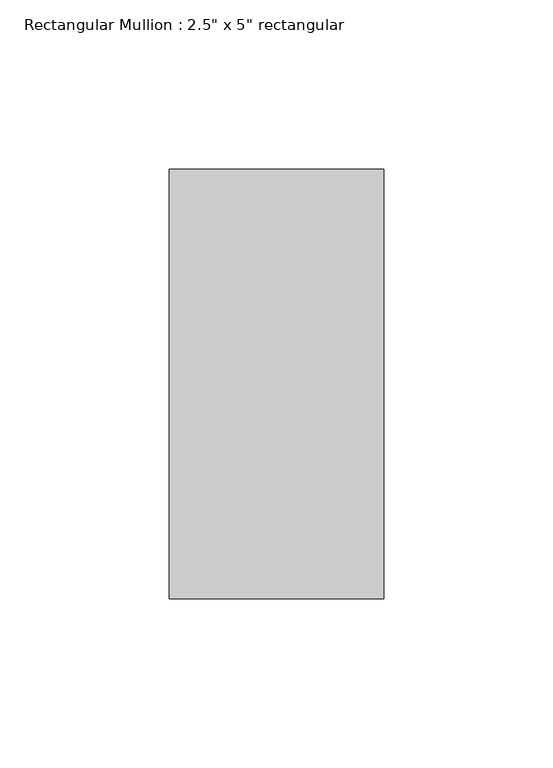
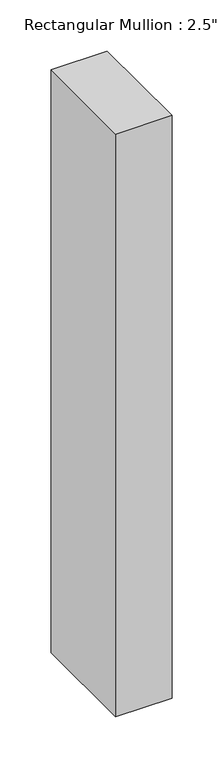
"""IFC4 building model written with IfcOpenShell, lengths in millimetres: member geometry."""

from ifc_helpers import new_model, si_unit, frame, origin, place, context, project, spatial, polyline, outline, extrude, source, transform, mapped, element, save


def member_b8383707(model_context):
    return source(origin(), model_context, "Body", "SweptSolid", [
        extrude(outline(polyline([(31.75, 63.5), (31.75, -63.5), (-31.75, -63.5), (-31.75, 63.5), (31.75, 63.5)])), frame((0.0, 0.0, -696.9443895), z_axis=(0.0, 0.0, 1.0), x_axis=(1.0, 0.0, 0.0)), (0.0, 0.0, 1.0), 696.9443895),
    ])


if __name__ == "__main__":
    model = new_model("IFC4")
    model_context = context("Model", 3, world=origin())
    ifc_project = project(units=[si_unit("LENGTHUNIT", "METRE", prefix="MILLI")], contexts=[model_context])
    site = spatial("IfcSite", under=ifc_project)
    building = spatial("IfcBuilding", under=site)
    placement = place(None, origin())
    member_shape = member_b8383707(model_context)
    element("IfcMember", 1, ObjectType="Rectangular Mullion : 2.5\" x 5\" rectangular", at=placement, inside=building, context=model_context, shape_type="MappedRepresentation", body=[
        mapped(member_shape, transform((0.0, 0.0, 0.0), x_axis=(1.0, 0.0, 0.0), y_axis=(0.0, 1.0, 0.0), z_axis=(0.0, 0.0, 1.0))),
    ])
    save(model, "model.ifc")

# Revit data of these elements
# Type "Rectangular Mullion : 2.5\" x 5\" rectangular"
#   built-in parameter 1007304 = 0.416667 (stored number, unit not read)
#   built-in parameter 1007301 = 0.104167 (stored number, unit not read)
#   built-in parameter 1007300 = 0.104167 (stored number, unit not read)
# Element 1 (IfcMember, "Rectangular Mullion : 2.5\" x 5\" rectangular")
#   Materials on its faces: "Aluminum"
# Materials
#   "Aluminum": class "Metal", colour RGB 247 247 247, transparency 0, Description = "Aluminum 6061", Cost = 0
